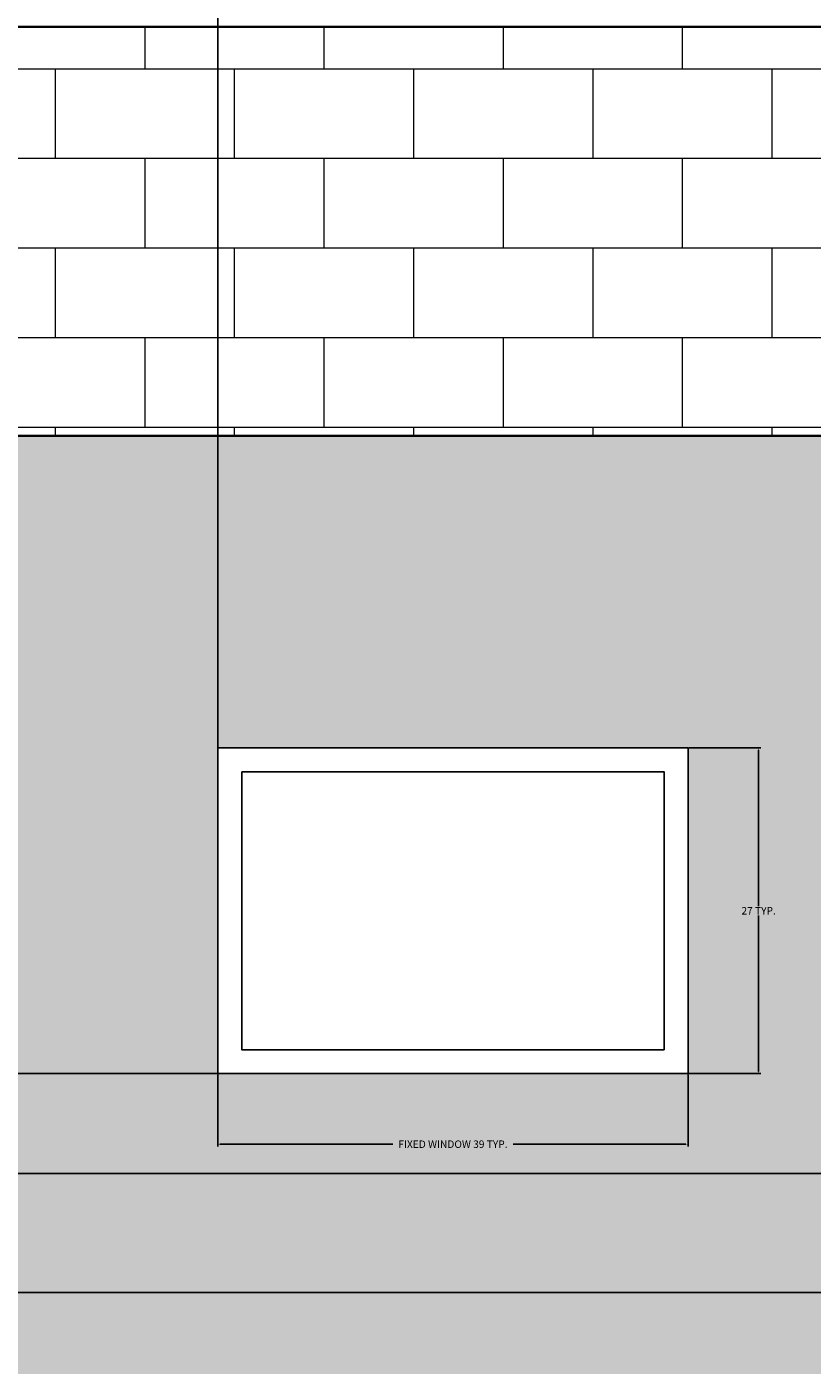
# Model space of a CAD drawing. Units: inches. Extents: x -13 to 809, y 112 to 656.
# Tile 38 of 55: x 455 to 521, y 446 to 559. Entities that reach past the tile are written whole.
import ezdxf

# ---------------------------------------------------------------- set-up
doc = ezdxf.new("R2010")
doc.units = ezdxf.units.IN
doc.header["$MEASUREMENT"] = 0
for name, color, linetype, lineweight in [('A-ANNO-DIMS', 2, 'Continuous', 18), ('A-ELEV', 7, 'Continuous', 35), ('A-ELEV-PATT', 8, 'Continuous', 13), ('A-GLAZ', 4, 'Continuous', 25)]:
    doc.layers.add(name, color=color, linetype=linetype, lineweight=lineweight)
doc.styles.get("Standard").update_dxf_attribs({"font": 'arial.ttf'})
doc.dimstyles.get("Standard").update_dxf_attribs({"dimtxt": 0.625, "dimasz": 0.18, "dimexe": 0.18, "dimexo": 0.0625, "dimgap": 0.09, "dimtad": 0, "dimtih": 1, "dimtoh": 1, "dimdec": 4, "dimzin": 0, "dimdsep": 46, "dimlunit": 4, "dimtxsty": 'Standard', "dimcen": 0.09, "dimadec": 0, "dimazin": 0, "dimtfac": 1, "dimtdec": 4, "dimtofl": 0, "dimtmove": 0, "dimatfit": 3, "dimfxl": 1, "dimtolj": 1, "dimtzin": 0, "dimarcsym": 0})

# ---------------------------------------------------------------- blocks, each defined once
blk = doc.blocks.new('WIN-FIXED-400')
for points in [[(0, 27.27), (39.36, 27.27), (39.36, 0), (0, 0)], [(2, 25.27), (37.36, 25.27), (37.36, 2), (2, 2)]]:
    blk.add_lwpolyline(points, close=True)
blk = doc.blocks.new('*D5')
at = {"layer": 'A-ANNO-DIMS', "color": 0, "lineweight": -2, "transparency": 16777216}
for p, q in [((471.1, 470.81), (471.1, 464.79)), ((510.46, 470.81), (510.46, 464.79)), ((471.28, 464.97), (485.74, 464.97)), ((510.28, 464.97), (495.82, 464.97))]:
    blk.add_line(p, q, dxfattribs=at)
at = {"layer": 'A-ANNO-DIMS', "color": 0, "transparency": 16777216}
for points in [[(471.28, 465), (471.28, 464.94), (471.1, 464.97)], [(510.28, 465), (510.28, 464.94), (510.46, 464.97)]]:
    blk.add_solid(points, dxfattribs=at)
at = {"layer": 'Defpoints', "color": 0, "transparency": 16777216}
for p in [(471.1, 470.88), (510.46, 470.88), (510.46, 464.97)]:
    blk.add_point(p, dxfattribs=at)
at = {"layer": 'A-ANNO-DIMS', "color": 0, "transparency": 16777216, "insert": (490.78, 464.97), "char_height": 0.625, "attachment_point": 5}
blk.add_mtext('\\A1;FIXED WINDOW 39 TYP.', dxfattribs=at)
blk = doc.blocks.new('*D6')
at = {"layer": 'A-ANNO-DIMS', "color": 0, "lineweight": -2, "transparency": 16777216}
for p, q in [((510.52, 498.15), (516.55, 498.15)), ((516.37, 497.97), (516.37, 484.91)), ((516.37, 471.06), (516.37, 484.11)), ((510.52, 470.88), (516.55, 470.88))]:
    blk.add_line(p, q, dxfattribs=at)
at = {"layer": 'A-ANNO-DIMS', "color": 0, "transparency": 16777216}
for points in [[(516.34, 497.97), (516.4, 497.97), (516.37, 498.15)], [(516.34, 471.06), (516.4, 471.06), (516.37, 470.88)]]:
    blk.add_solid(points, dxfattribs=at)
at = {"layer": 'Defpoints', "color": 0, "transparency": 16777216}
for p in [(510.46, 498.15), (516.37, 498.15), (510.46, 470.88)]:
    blk.add_point(p, dxfattribs=at)
at = {"layer": 'A-ANNO-DIMS', "color": 0, "transparency": 16777216, "insert": (516.37, 484.51), "char_height": 0.625, "attachment_point": 5}
blk.add_mtext('\\A1;27 TYP.', dxfattribs=at)
blk = doc.blocks.new('*D26')
at = {"layer": 'A-ANNO-DIMS', "color": 0, "lineweight": -2, "transparency": 16777216}
for p, q in [((341.41, 524.34), (341.41, 655.96)), ((341.59, 655.78), (405.14, 655.78)), ((470.92, 655.78), (407.37, 655.78)), ((471.1, 470.94), (471.1, 655.96))]:
    blk.add_line(p, q, dxfattribs=at)
at = {"layer": 'A-ANNO-DIMS', "color": 0, "transparency": 16777216}
for points in [[(341.59, 655.81), (341.59, 655.75), (341.41, 655.78)], [(470.92, 655.81), (470.92, 655.75), (471.1, 655.78)]]:
    blk.add_solid(points, dxfattribs=at)
at = {"layer": 'Defpoints', "color": 0, "transparency": 16777216}
for p in [(471.1, 655.78), (341.41, 524.28), (471.1, 470.88)]:
    blk.add_point(p, dxfattribs=at)
at = {"layer": 'A-ANNO-DIMS', "color": 0, "transparency": 16777216, "insert": (406.25, 655.78), "char_height": 0.625, "attachment_point": 5}
blk.add_mtext('\\A1;129.7', dxfattribs=at)
blk = doc.blocks.new('*D27')
at = {"layer": 'A-ANNO-DIMS', "color": 0, "lineweight": -2, "transparency": 16777216}
for p, q in [((471.1, 470.94), (471.1, 655.96)), ((471.28, 655.78), (505.89, 655.78)), ((542.78, 655.78), (508.17, 655.78)), ((542.96, 524.34), (542.96, 655.96))]:
    blk.add_line(p, q, dxfattribs=at)
at = {"layer": 'A-ANNO-DIMS', "color": 0, "transparency": 16777216}
for points in [[(471.28, 655.81), (471.28, 655.75), (471.1, 655.78)], [(542.78, 655.81), (542.78, 655.75), (542.96, 655.78)]]:
    blk.add_solid(points, dxfattribs=at)
at = {"layer": 'Defpoints', "color": 0, "transparency": 16777216}
for p in [(542.96, 655.78), (542.96, 524.28), (471.1, 470.88)]:
    blk.add_point(p, dxfattribs=at)
at = {"layer": 'A-ANNO-DIMS', "color": 0, "transparency": 16777216, "insert": (507.03, 655.78), "char_height": 0.625, "attachment_point": 5}
blk.add_mtext('\\A1;71.86', dxfattribs=at)
blk = doc.blocks.new('*D43')
at = {"layer": 'A-ANNO-DIMS', "color": 0, "lineweight": -2, "transparency": 16777216}
for p, q in [((471.04, 470.88), (-12.1, 470.88)), ((-11.92, 470.7), (-11.92, 443.28)), ((-11.92, 415.04), (-11.92, 442.46)), ((471.04, 414.86), (-12.1, 414.86))]:
    blk.add_line(p, q, dxfattribs=at)
at = {"layer": 'A-ANNO-DIMS', "color": 0, "transparency": 16777216}
for points in [[(-11.95, 470.7), (-11.89, 470.7), (-11.92, 470.88)], [(-11.95, 415.04), (-11.89, 415.04), (-11.92, 414.86)]]:
    blk.add_solid(points, dxfattribs=at)
at = {"layer": 'Defpoints', "color": 0, "transparency": 16777216}
for p in [(-11.92, 470.88), (471.1, 470.88), (471.1, 414.86)]:
    blk.add_point(p, dxfattribs=at)
at = {"layer": 'A-ANNO-DIMS', "color": 0, "transparency": 16777216, "insert": (-11.92, 442.87), "char_height": 0.625, "attachment_point": 5}
blk.add_mtext('\\A1;56.02', dxfattribs=at)
blk = doc.blocks.new('*D104')
at = {"layer": 'A-ANNO-DIMS', "color": 0, "lineweight": -2, "transparency": 16777216}
for p, q in [((337.57, 462.52), (807.77, 462.52)), ((807.59, 462.34), (807.59, 457.95)), ((807.59, 452.74), (807.59, 457.13)), ((319.76, 452.56), (807.77, 452.56))]:
    blk.add_line(p, q, dxfattribs=at)
at = {"layer": 'A-ANNO-DIMS', "color": 0, "transparency": 16777216}
for points in [[(807.56, 462.34), (807.62, 462.34), (807.59, 462.52)], [(807.56, 452.74), (807.62, 452.74), (807.59, 452.56)]]:
    blk.add_solid(points, dxfattribs=at)
at = {"layer": 'Defpoints', "color": 0, "transparency": 16777216}
for p in [(337.51, 462.52), (319.7, 452.56), (807.59, 452.56)]:
    blk.add_point(p, dxfattribs=at)
at = {"layer": 'A-ANNO-DIMS', "color": 0, "transparency": 16777216, "insert": (807.59, 457.54), "char_height": 0.625, "attachment_point": 5}
blk.add_mtext('\\A1;9.957', dxfattribs=at)
blk = doc.blocks.new('*D105')
at = {"layer": 'A-ANNO-DIMS', "color": 0, "lineweight": -2, "transparency": 16777216}
for p, q in [((319.76, 452.56), (807.77, 452.56)), ((807.59, 452.38), (807.59, 448.95)), ((807.59, 444.7), (807.59, 448.13)), ((319.57, 444.52), (807.77, 444.52))]:
    blk.add_line(p, q, dxfattribs=at)
at = {"layer": 'A-ANNO-DIMS', "color": 0, "transparency": 16777216}
for points in [[(807.56, 452.38), (807.62, 452.38), (807.59, 452.56)], [(807.56, 444.7), (807.62, 444.7), (807.59, 444.52)]]:
    blk.add_solid(points, dxfattribs=at)
at = {"layer": 'Defpoints', "color": 0, "transparency": 16777216}
for p in [(319.7, 452.56), (319.51, 444.52), (807.59, 444.52)]:
    blk.add_point(p, dxfattribs=at)
at = {"layer": 'A-ANNO-DIMS', "color": 0, "transparency": 16777216, "insert": (807.59, 448.54), "char_height": 0.625, "attachment_point": 5}
blk.add_mtext('\\A1;8.043', dxfattribs=at)

msp = doc.modelspace()

# ---------------------------------------------------------------- hatches: boundary and pattern name
at = {"layer": 'A-ELEV-PATT'}
h = msp.add_hatch(dxfattribs=at)
h.set_pattern_fill('BRICK', color=256, scale=30)
h.paths.add_polyline_path([(591.008, 558.5199), (341.4072, 558.5199), (341.4072, 524.281), (542.9617, 524.281), (542.9617, 288.4508), (341.4072, 288.4508), (341.4072, 250.8429), (591.008, 250.8429)])
h = msp.add_hatch(dxfattribs=at)
h.set_pattern_fill('CROSS', color=256, scale=9.7)
h.paths.add_polyline_path([(542.9617, 524.281), (442.1845, 524.281), (442.1845, 288.4508), (542.9617, 288.4508)])
h.paths.add_polyline_path([(471.0998, 470.8765), (471.0998, 498.1452), (510.462, 498.1452), (510.462, 470.8765)], flags=16)
h.paths.add_polyline_path([(473.0998, 472.8765), (473.0998, 496.1452), (508.462, 496.1452), (508.462, 472.8765)], flags=0)
h.paths.add_polyline_path([(471.0998, 442.128), (510.462, 442.128), (510.462, 414.8594), (471.0998, 414.8594)], flags=16)
h.paths.add_polyline_path([(473.0998, 440.128), (508.462, 440.128), (508.462, 416.8594), (473.0998, 416.8594)], flags=0)
h.paths.add_polyline_path([(471.0998, 385.2491), (510.462, 385.2491), (510.462, 357.9804), (471.0998, 357.9804)], flags=16)
h.paths.add_polyline_path([(473.0998, 383.2491), (508.462, 383.2491), (508.462, 359.9804), (473.0998, 359.9804)], flags=0)
h.paths.add_polyline_path([(471.0998, 340.4353), (510.462, 340.4353), (510.462, 313.1667), (471.0998, 313.1667)], flags=16)
h.paths.add_polyline_path([(473.0998, 338.4353), (508.462, 338.4353), (508.462, 315.1667), (473.0998, 315.1667)], flags=0)

# ---------------------------------------------------------------- linework, layer by layer
at = {"layer": 'A-ELEV'}
msp.add_line((341.4072, 558.5199), (591.008, 558.5199), dxfattribs=at)
for points in [[(341.4072, 558.5199), (591.008, 558.5199), (591.008, 250.8429), (341.4072, 250.8429)], [(341.4072, 524.281), (542.9617, 524.281), (542.9617, 288.4508), (341.4072, 288.4508)]]:
    msp.add_lwpolyline(points, close=True, dxfattribs=at)

# ---------------------------------------------------------------- block references
at = {"layer": 'A-GLAZ'}
msp.add_blockref('WIN-FIXED-400', (471.1, 470.877), dxfattribs=at)

# ---------------------------------------------------------------- dimensions: what is measured, and where the dimension line sits
at = {"layer": 'A-ANNO-DIMS'}
for base, p1, p2, override, picture, middle in [((471.0998, 655.7828), (341.4072, 524.281), (471.0998, 470.8765), {"dimdec": 1, "dimlfac": 1, "dimrnd": 0, "dimzin": 0, "dimdsep": 46, "dimlunit": 2}, '*D26', (406.2535, 655.7828)), ((542.9617, 655.7828), (471.0998, 470.8765), (542.9617, 524.281), {"dimdec": 2, "dimlfac": 1, "dimrnd": 0, "dimzin": 0, "dimdsep": 46, "dimlunit": 2}, '*D27', (507.0308, 655.7828))]:
    dim = msp.add_linear_dim(base=base, p1=p1, p2=p2, dimstyle='Standard', override=override, dxfattribs=at)
    dim.commit()
    dim.dimension.update_dxf_attribs({"geometry": picture, "text_midpoint": middle})
dim = msp.add_linear_dim(base=(516.3663, 498.1452), p1=(510.462, 470.8765), p2=(510.462, 498.1452), angle=90, text='<> TYP.', dimstyle='Standard', override={"dimdec": 0, "dimlfac": 1, "dimrnd": 0, "dimzin": 0, "dimdsep": 46, "dimlunit": 2}, dxfattribs=at)
dim.commit()
dim.dimension.update_dxf_attribs({"geometry": '*D6', "text_midpoint": (516.3663, 484.5108)})
for base, p1, p2, override, picture, middle in [((-11.9191, 470.8765), (471.0998, 414.8594), (471.0998, 470.8765), {"dimdec": 2, "dimlfac": 1, "dimrnd": 0, "dimzin": 0, "dimdsep": 46, "dimlunit": 2}, '*D43', (-11.9191, 442.8679)), ((807.5888, 452.5629), (337.5074, 462.5199), (319.7004, 452.5629), {"dimdec": 3, "dimlfac": 1, "dimrnd": 0, "dimzin": 0, "dimdsep": 46, "dimlunit": 2}, '*D104', (807.5888, 457.5414)), ((807.5888, 444.5199), (319.7004, 452.5629), (319.5074, 444.5199), {"dimdec": 3, "dimlfac": 1, "dimrnd": 0, "dimzin": 0, "dimdsep": 46, "dimlunit": 2}, '*D105', (807.5888, 448.5414))]:
    dim = msp.add_linear_dim(base=base, p1=p1, p2=p2, angle=90, dimstyle='Standard', override=override, dxfattribs=at)
    dim.commit()
    dim.dimension.update_dxf_attribs({"geometry": picture, "text_midpoint": middle})
dim = msp.add_linear_dim(base=(510.462, 464.9722), p1=(471.0998, 470.8765), p2=(510.462, 470.8765), text='FIXED WINDOW <> TYP.', dimstyle='Standard', override={"dimdec": 0, "dimlfac": 1, "dimrnd": 0, "dimzin": 0, "dimdsep": 46, "dimlunit": 2}, dxfattribs=at)
dim.commit()
dim.dimension.update_dxf_attribs({"geometry": '*D5', "text_midpoint": (490.7809, 464.9722)})

doc.saveas('drawing.dxf')
